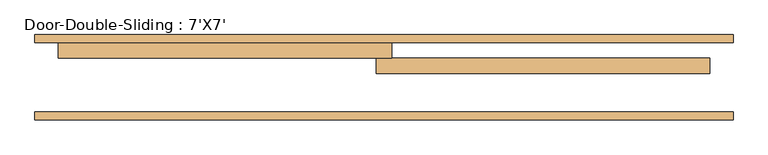
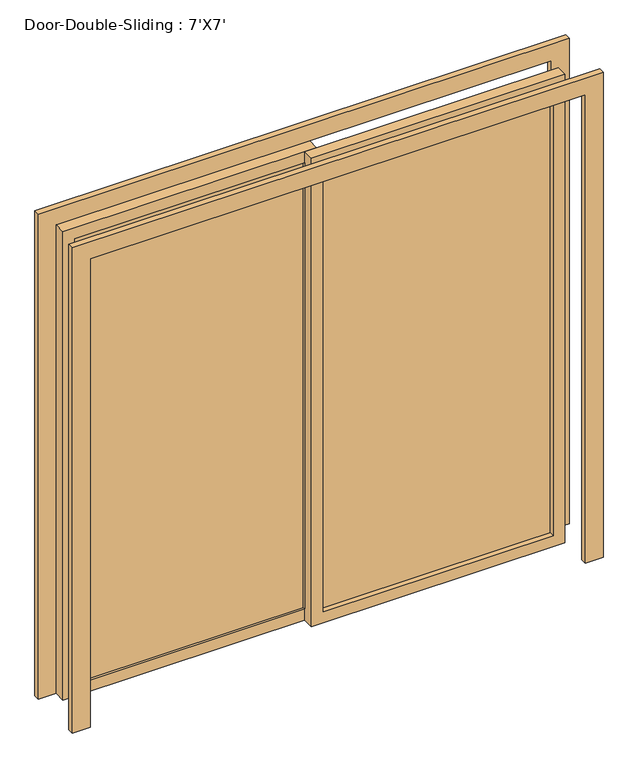
"""IFC4 building model written with IfcOpenShell, lengths in millimetres: door geometry, Door-Double-Sliding : 7'X7'."""

from ifc_helpers import new_model, si_unit, frame, origin, place, context, project, spatial, polyline, outline, extrude, source, transform, mapped, element, save


def door_double_sliding_7_x7_ddbaaa7c(model_context):
    return source(origin(), model_context, "Body", "SweptSolid", [
        extrude(outline(polyline([(0.0, 1143.0), (2209.8, 1143.0), (2209.8, -1143.0), (0.0, -1143.0), (0.0, -1066.8), (2133.6, -1066.8), (2133.6, 1066.8), (0.0, 1066.8), (0.0, 1143.0)])), frame((0.0, 241.3, 0.0), z_axis=(0.0, 1.0, 0.0), x_axis=(0.0, 0.0, 1.0)), (0.0, 0.0, 1.0), 25.4),
        extrude(outline(polyline([(0.0, -1143.0), (0.0, -1066.8), (2133.6, -1066.8), (2133.6, 1066.8), (0.0, 1066.8), (0.0, 1143.0), (2209.8, 1143.0), (2209.8, -1143.0), (0.0, -1143.0)])), frame((0.0, -12.7, 0.0), z_axis=(0.0, 1.0, 0.0), x_axis=(0.0, 0.0, 1.0)), (0.0, 0.0, 1.0), 25.4),
        extrude(outline(polyline([(2133.6, 25.4), (2133.6, -1066.8), (0.0, -1066.8), (0.0, 25.4), (2133.6, 25.4)]), holes=[polyline([(2082.8, -25.4), (50.8, -25.4), (50.8, -1016.0), (2082.8, -1016.0), (2082.8, -25.4)])]), frame((0.0, 190.5, 0.0), z_axis=(0.0, 1.0, 0.0), x_axis=(0.0, 0.0, 1.0)), (0.0, 0.0, 1.0), 50.8),
        extrude(outline(polyline([(2133.6, -25.4), (0.0, -25.4), (0.0, 1066.8), (2133.6, 1066.8), (2133.6, -25.4)]), holes=[polyline([(2082.8, 25.4), (2082.8, 1016.0), (50.8, 1016.0), (50.8, 25.4), (2082.8, 25.4)])]), frame((0.0, 139.7, 0.0), z_axis=(0.0, 1.0, 0.0), x_axis=(0.0, 0.0, 1.0)), (0.0, 0.0, 1.0), 50.8),
        extrude(outline(polyline([(-25.4, 200.025), (-1016.0, 200.025), (-1016.0, 206.375), (-25.4, 206.375), (-25.4, 200.025)])), frame((0.0, 0.0, 50.8), z_axis=(0.0, 0.0, 1.0), x_axis=(1.0, 0.0, 0.0)), (0.0, 0.0, 1.0), 2032.0),
        extrude(outline(polyline([(25.4, 168.275), (1016.0, 168.275), (1016.0, 161.925), (25.4, 161.925), (25.4, 168.275)])), frame((0.0, 0.0, 50.8), z_axis=(0.0, 0.0, 1.0), x_axis=(1.0, 0.0, 0.0)), (0.0, 0.0, 1.0), 2032.0),
    ])


if __name__ == "__main__":
    model = new_model("IFC4")
    model_context = context("Model", 3, world=origin())
    ifc_project = project(units=[si_unit("LENGTHUNIT", "METRE", prefix="MILLI")], contexts=[model_context])
    site = spatial("IfcSite", under=ifc_project)
    building = spatial("IfcBuilding", under=site)
    placement = place(None, origin())
    door_double_sliding_7_x7_shape = door_double_sliding_7_x7_ddbaaa7c(model_context)
    element("IfcDoor", 1, ObjectType="Door-Double-Sliding : 7'X7'", at=placement, inside=building, context=model_context, shape_type="MappedRepresentation", body=[
        mapped(door_double_sliding_7_x7_shape, transform((0.0, 0.0, 0.0), x_axis=(1.0, 0.0, 0.0), y_axis=(0.0, 1.0, 0.0), z_axis=(0.0, 0.0, 1.0))),
    ])
    save(model, "model.ifc")

# Revit data of these elements
# Type "Door-Double-Sliding : 7'X7'"
#   Type Mark = "14"
#   Construction Type Id = "opn-d45"
#   Assembly Code = "C1020"
#   Analytic Construction = "Wood frame, double glass door "
#   Thickness = 0' - 2"
#   Thermal Resistance (R) = 1.8150 (h·ft²·°F)/BTU
#   Heat Transfer Coefficient (U) = 0.5510 BTU/(h·ft²·°F)
#   Height = 7' - 0"
#   Rail Width = 0' - 2"
#   Stiles = 0' - 2"
#   Trim Projection Ext = 0' - 1"
#   Trim Projection Int = 0' - 1"
#   Trim Width = 0' - 3"
#   Width = 7' - 0"
#   Define Thermal Properties by = 1
#   Glazing = Glass
#   Panel Material = Wood - Birch - Solid Stained Light Low Gloss
#   Trim Material = Paint - Sienna
#   Visual Light Transmittance = 0
#   Solar Heat Gain Coefficient = 0
#   Function = (empty or 0)
#   Wall Closure = (empty or 0)
# Element 1 (IfcDoor, "Door-Double-Sliding : 7'X7'")
#   Materials on its faces: "Paint - Sienna", "Wood - Birch - Solid Stained Light Low Gloss", "Glass"
# Materials
#   "Glass": class "Glass", colour RGB 0 128 192, transparency 0.75, Description = "Soda Lime Glass", Cost = 0
#   "Wood - Birch - Solid Stained Light Low Gloss": class "Wood", colour RGB 210 159 95, transparency 0, Cost = 0
#   "Paint - Sienna": colour RGB 118 70 51, transparency 0, Cost = 0
